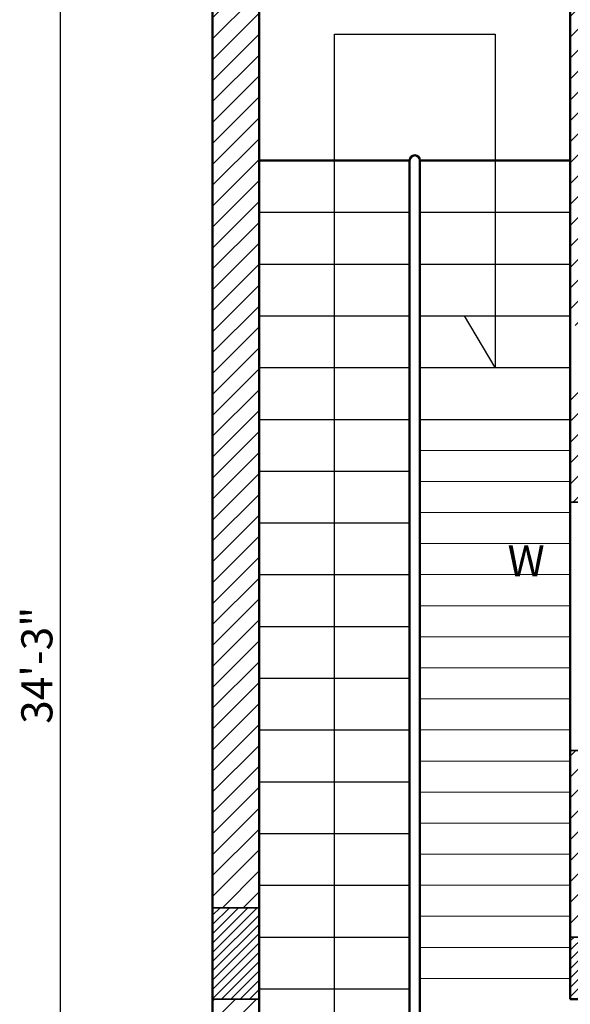
# Model space of a CAD drawing. Units: millimetres. Extents: x 225995 to 227247, y 225507 to 226008.
# Tile 12 of 23: x 226643 to 226749, y 225691 to 225881. Entities that reach past the tile are written whole.
import ezdxf

# ---------------------------------------------------------------- set-up
doc = ezdxf.new("R2010")
doc.units = ezdxf.units.MM
for name, color, linetype, lineweight in [('A-ANNO-DIMS', 2, 'Continuous', 18), ('A-ANNO-TEXT', 3, 'Continuous', 18), ('A-COLS', 40, 'Continuous', 35), ('A-FLOR-PATT', 8, 'Continuous', 13), ('A-FLOR-STRS', 141, 'Continuous', 25), ('A-GLAZ', 4, 'Continuous', 25), ('A-WALL', 7, 'Continuous', 50), ('A-WALL-PATT', 8, 'Continuous', 13)]:
    doc.layers.add(name, color=color, linetype=linetype, lineweight=lineweight)
doc.styles.get("Standard").update_dxf_attribs({"font": 'arial.ttf'})
doc.dimstyles.new('ISO-25', dxfattribs={"dimtxt": 6, "dimasz": 2.5, "dimexe": 1.25, "dimexo": 0.625, "dimtad": 1, "dimdec": 0, "dimlunit": 3, "dimtxsty": 'Standard', "dimcen": 2.5, "dimadec": 0, "dimazin": 0, "dimtfac": 1, "dimtdec": 0, "dimtmove": 0, "dimatfit": 3, "dimfxl": 1, "dimarcsym": 0})
pattern_1 = [(45, (646.0463, 0.931), (-2.020557627, 2.020557627), [])]

# ---------------------------------------------------------------- blocks, each defined once
blk = doc.blocks.new('*D113')
at = {"layer": 'A-ANNO-DIMS', "color": 0, "lineweight": -2, "transparency": 16777216}
for p, q in [((226679.3, 225961.7), (226649.22, 225961.7)), ((226650.47, 225959.2), (226650.47, 225553.2)), ((226679.3, 225550.7), (226649.22, 225550.7))]:
    blk.add_line(p, q, dxfattribs=at)
at = {"layer": 'A-ANNO-DIMS', "color": 0, "transparency": 16777216}
for points in [[(226650.06, 225959.2), (226650.89, 225959.2), (226650.47, 225961.7)], [(226650.06, 225553.2), (226650.89, 225553.2), (226650.47, 225550.7)]]:
    blk.add_solid(points, dxfattribs=at)
at = {"layer": 'Defpoints', "color": 0, "transparency": 16777216}
for p in [(226679.92, 225961.7), (226650.47, 225550.7), (226679.92, 225550.7)]:
    blk.add_point(p, dxfattribs=at)
at = {"layer": 'A-ANNO-DIMS', "color": 0, "transparency": 16777216, "insert": (226646.78, 225756.2), "char_height": 6, "attachment_point": 5, "rotation": 90}
blk.add_mtext('34\'-3"', dxfattribs=at)

msp = doc.modelspace()

# ---------------------------------------------------------------- hatches: boundary and pattern name
at = {"layer": 'A-WALL-PATT'}
h = msp.add_hatch(dxfattribs=at)
h.set_pattern_fill('ANSI31', color=256, scale=0.9)
h.set_pattern_definition(pattern_1)
h.paths.add_polyline_path([(226757.92, 225925.7), (226748.92, 225925.7), (226748.92, 225904.7), (226742.92, 225904.7), (226742.92, 225895.7), (226748.92, 225895.7), (226748.92, 225821.85), (226757.92, 225821.85)])
h = msp.add_hatch(dxfattribs=at)
h.set_pattern_fill('ANSI31', color=256, scale=0.9)
h.set_pattern_definition(pattern_1)
h.paths.add_polyline_path([(226688.92, 225895.61), (226679.92, 225895.61), (226679.92, 225709.35), (226688.92, 225709.35)])
h = msp.add_hatch(dxfattribs=at)
h.set_pattern_fill('ANSI31', color=256, scale=0.9)
h.paths.add_polyline_path([(226757.92, 225809.85), (226748.92, 225809.85), (226748.92, 225787.7), (226757.92, 225787.7)])
h = msp.add_hatch(dxfattribs=at)
h.set_pattern_fill('ANSI31', color=256, scale=0.9)
h.paths.add_polyline_path([(226757.92, 225739.7), (226748.92, 225739.7), (226748.92, 225703.7), (226757.92, 225703.7)])
h = msp.add_hatch(dxfattribs=at)
h.set_pattern_fill('ANSI31', color=256, scale=0.4)
h.set_pattern_definition([(45, (646.0463, 0.931), (-0.898025612, 0.898025612), [])])
h.paths.add_polyline_path([(226688.92, 225709.35), (226679.92, 225709.35), (226679.92, 225691.7), (226688.92, 225691.7)])
h = msp.add_hatch(dxfattribs=at)
h.set_pattern_fill('ANSI31', color=256, scale=0.4)
h.set_pattern_definition([(45, (646.0463, 120.931), (-0.898025612, 0.898025612), [])])
h.paths.add_polyline_path([(226757.92, 225703.7), (226748.92, 225703.7), (226748.92, 225691.7), (226757.92, 225691.7)])
h = msp.add_hatch(dxfattribs=at)
h.set_pattern_fill('ANSI31', color=256, scale=0.9)
h.set_pattern_definition(pattern_1)
h.paths.add_polyline_path([(226688.92, 225691.7), (226679.92, 225691.7), (226679.92, 225673.7), (226688.92, 225673.7)])

# ---------------------------------------------------------------- linework, layer by layer
at = {"layer": 'A-COLS'}
for p, q in [((226757.92, 225787.7), (226748.92, 225787.7)), ((226757.92, 225739.7), (226748.92, 225739.7))]:
    msp.add_line(p, q, dxfattribs=at)
for points in [[(226688.92, 225691.7), (226679.92, 225691.7), (226679.92, 225709.35), (226688.92, 225709.35)], [(226757.92, 225691.7), (226748.92, 225691.7), (226748.92, 225703.7), (226757.92, 225703.7)]]:
    msp.add_lwpolyline(points, close=True, dxfattribs=at)
at = {"layer": 'A-FLOR-PATT'}
for p, q in [((226748.92, 225797.7), (226719.92, 225797.7)), ((226748.92, 225791.7), (226719.92, 225791.7)), ((226748.92, 225785.7), (226719.92, 225785.7)), ((226748.92, 225779.7), (226719.92, 225779.7)), ((226748.92, 225773.7), (226719.92, 225773.7)), ((226748.92, 225767.7), (226719.92, 225767.7)), ((226748.92, 225761.7), (226719.92, 225761.7)), ((226748.92, 225755.7), (226719.92, 225755.7)), ((226748.92, 225749.7), (226719.92, 225749.7)), ((226748.92, 225743.7), (226719.92, 225743.7)), ((226748.92, 225737.7), (226719.92, 225737.7)), ((226748.92, 225731.7), (226719.92, 225731.7)), ((226748.92, 225725.7), (226719.92, 225725.7)), ((226748.92, 225719.7), (226719.92, 225719.7)), ((226748.92, 225713.7), (226719.92, 225713.7)), ((226748.92, 225707.7), (226719.92, 225707.7)), ((226748.92, 225701.7), (226719.92, 225701.7)), ((226748.92, 225695.7), (226719.92, 225695.7))]:
    msp.add_line(p, q, dxfattribs=at)
at = {"layer": 'A-FLOR-STRS'}
for p, q in [((226703.42, 225673.7), (226703.42, 225878.09)), ((226703.42, 225878.09), (226734.42, 225878.09)), ((226734.42, 225878.09), (226734.42, 225813.7)), ((226688.92, 225843.7), (226717.92, 225843.7)), ((226719.92, 225843.7), (226748.92, 225843.7)), ((226688.92, 225833.7), (226717.92, 225833.7)), ((226719.92, 225833.7), (226748.92, 225833.7)), ((226688.92, 225823.7), (226717.92, 225823.7)), ((226719.92, 225823.7), (226748.92, 225823.7)), ((226734.42, 225813.7), (226728.51, 225823.7)), ((226728.51, 225823.7), (226734.42, 225823.7)), ((226688.92, 225813.7), (226717.92, 225813.7)), ((226719.92, 225813.7), (226748.92, 225813.7)), ((226688.92, 225803.7), (226717.92, 225803.7)), ((226719.92, 225803.7), (226748.92, 225803.7)), ((226688.92, 225793.7), (226717.92, 225793.7)), ((226688.92, 225783.7), (226717.92, 225783.7)), ((226688.92, 225773.7), (226717.92, 225773.7)), ((226688.92, 225763.7), (226717.92, 225763.7)), ((226688.92, 225753.7), (226717.92, 225753.7)), ((226688.92, 225743.7), (226717.92, 225743.7)), ((226688.92, 225733.7), (226717.92, 225733.7)), ((226688.92, 225723.7), (226717.92, 225723.7)), ((226688.92, 225713.7), (226717.92, 225713.7)), ((226688.92, 225703.7), (226717.92, 225703.7)), ((226688.92, 225693.7), (226717.92, 225693.7))]:
    msp.add_line(p, q, dxfattribs=at)
at = {"layer": 'A-GLAZ'}
msp.add_lwpolyline([(226748.92, 225787.7), (226757.92, 225787.7), (226757.92, 225739.7), (226748.92, 225739.7)], close=True, dxfattribs=at)
at = {"layer": 'A-WALL'}
for p, q in [((226679.92, 225673.7), (226679.92, 225961.7)), ((226679.92, 225673.7), (226679.92, 225961.7)), ((226688.92, 225673.7), (226688.92, 225895.7)), ((226688.92, 225895.61), (226688.92, 225673.7)), ((226748.92, 225691.7), (226748.92, 225895.7)), ((226748.92, 225691.7), (226748.92, 225895.7)), ((226688.92, 225853.7), (226717.92, 225853.7)), ((226717.92, 225853.7), (226717.92, 225673.7)), ((226719.92, 225853.7), (226748.92, 225853.7)), ((226719.92, 225853.7), (226719.92, 225673.7)), ((226748.92, 225691.7), (226889.92, 225691.7)), ((226880.92, 225691.7), (226748.92, 225691.7))]:
    msp.add_line(p, q, dxfattribs=at)
msp.add_arc((226718.92, 225853.7), 1, 0, 180, dxfattribs=at)

# ---------------------------------------------------------------- texts
at = {"layer": 'A-ANNO-TEXT', "insert": (226731.31, 225779.38), "char_height": 6, "attachment_point": 1}
msp.add_mtext_dynamic_manual_height_columns('   W', width=24.8115, gutter_width=12.5, heights=[0], dxfattribs=at)

# ---------------------------------------------------------------- dimensions: what is measured, and where the dimension line sits
at = {"layer": 'A-ANNO-DIMS'}
dim = msp.add_linear_dim(base=(226650.47, 225550.7), p1=(226679.92, 225961.7), p2=(226679.92, 225550.7), angle=90, dimstyle='ISO-25', override={"dimdec": 1, "dimlfac": 1, "dimrnd": 0, "dimzin": 1, "dimdsep": 46, "dimlunit": 4, "dimfrac": 2}, dxfattribs=at)
dim.commit()
dim.dimension.update_dxf_attribs({"geometry": '*D113', "text_midpoint": (226646.78, 225756.2)})

doc.saveas('drawing.dxf')
